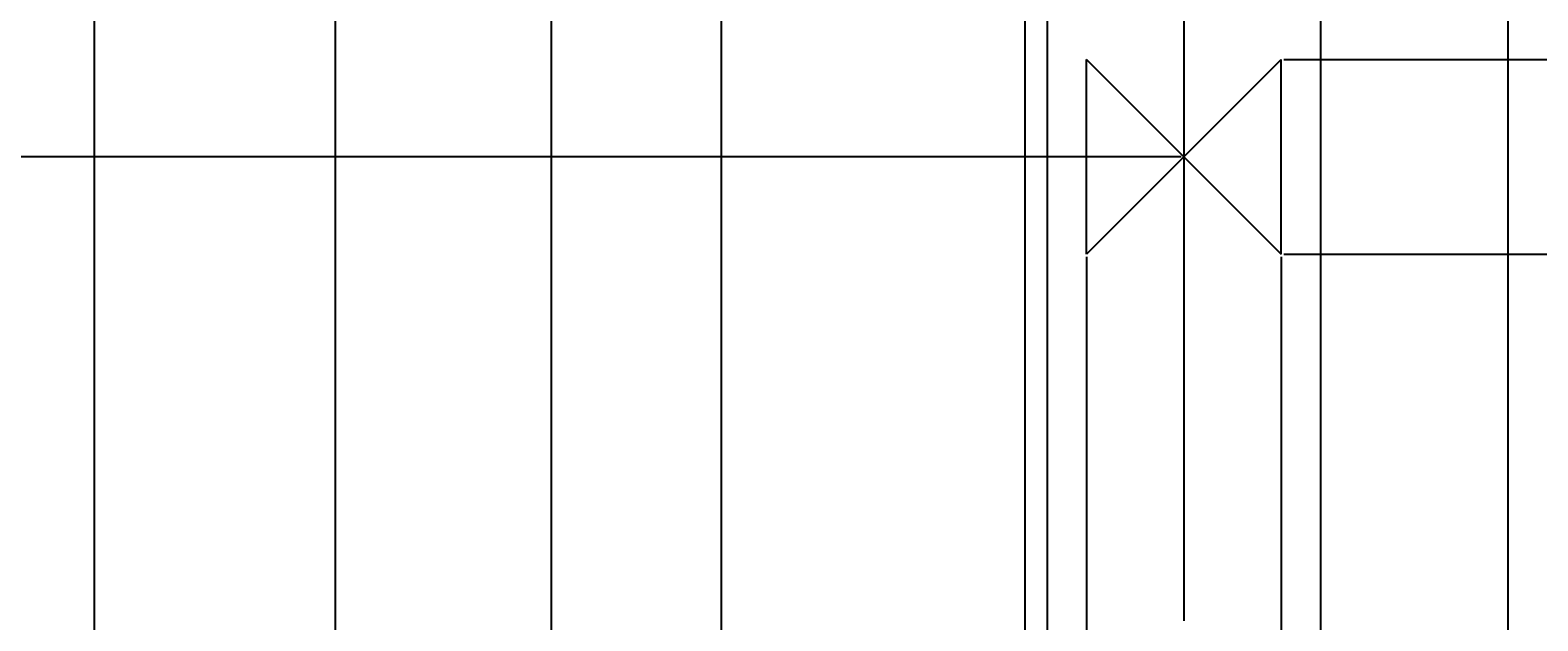
# Model space of a CAD drawing. Units: inches. Extents: x 412 to 584, y 208 to 437.
# Tile 18 of 28: x 471 to 508, y 338 to 352. Entities that reach past the tile are written whole.
import ezdxf

# ---------------------------------------------------------------- set-up
doc = ezdxf.new("R2010")
doc.units = ezdxf.units.IN
doc.header["$MEASUREMENT"] = 0
doc.layers.add('A-ANNO-DIMS', color=2, linetype='Continuous', lineweight=18)
doc.layers.add('E-POWR-EQPM', color=3, linetype='Continuous', lineweight=25)
doc.styles.get("Standard").update_dxf_attribs({"font": 'arial.ttf'})
doc.dimstyles.get("Standard").update_dxf_attribs({"dimtxt": 0.18, "dimasz": 0.18, "dimexe": 0.18, "dimexo": 0.0625, "dimgap": 0.09, "dimtad": 0, "dimtih": 1, "dimtoh": 1, "dimdec": 4, "dimzin": 0, "dimdsep": 46, "dimtxsty": 'Standard', "dimcen": 0.09, "dimadec": 0, "dimazin": 0, "dimtfac": 1, "dimtdec": 4, "dimtofl": 0, "dimtmove": 0, "dimatfit": 3, "dimfxl": 1, "dimtolj": 1, "dimtzin": 0, "dimarcsym": 0})

# ---------------------------------------------------------------- blocks, each defined once
blk = doc.blocks.new('*D17')
at = {"layer": 'A-ANNO-DIMS', "color": 0, "lineweight": -2, "transparency": 16777216}
for p, q in [((497.715, 426.185), (583.674, 426.185)), ((583.494, 426.005), (583.494, 323.031)), ((583.494, 219.693), (583.494, 322.667)), ((550.198, 219.513), (583.674, 219.513))]:
    blk.add_line(p, q, dxfattribs=at)
at = {"layer": 'A-ANNO-DIMS', "color": 0, "transparency": 16777216}
for points in [[(583.464, 426.005), (583.524, 426.005), (583.494, 426.185)], [(583.464, 219.693), (583.524, 219.693), (583.494, 219.513)]]:
    blk.add_solid(points, dxfattribs=at)
at = {"layer": 'Defpoints', "color": 0, "transparency": 16777216}
for p in [(497.652, 426.185), (550.135, 219.513), (583.494, 219.513)]:
    blk.add_point(p, dxfattribs=at)
at = {"layer": 'A-ANNO-DIMS', "color": 0, "transparency": 16777216, "insert": (583.494, 322.849), "char_height": 0.18, "attachment_point": 5}
blk.add_mtext('\\A1;206.67', dxfattribs=at)
blk = doc.blocks.new('*D23')
at = {"layer": 'A-ANNO-DIMS', "color": 0, "lineweight": -2, "transparency": 16777216}
for p, q in [((466.041, 360.196), (412.276, 360.196)), ((412.456, 360.016), (412.456, 354.967)), ((412.456, 349.553), (412.456, 354.603)), ((499.225, 349.373), (412.276, 349.373))]:
    blk.add_line(p, q, dxfattribs=at)
at = {"layer": 'A-ANNO-DIMS', "color": 0, "transparency": 16777216}
for points in [[(412.426, 360.016), (412.486, 360.016), (412.456, 360.196)], [(412.426, 349.553), (412.486, 349.553), (412.456, 349.373)]]:
    blk.add_solid(points, dxfattribs=at)
at = {"layer": 'Defpoints', "color": 0, "transparency": 16777216}
for p in [(466.104, 360.196), (412.456, 349.373), (499.288, 349.373)]:
    blk.add_point(p, dxfattribs=at)
at = {"layer": 'A-ANNO-DIMS', "color": 0, "transparency": 16777216, "insert": (412.456, 354.785), "char_height": 0.18, "attachment_point": 5}
blk.add_mtext('\\A1;10.823', dxfattribs=at)
blk = doc.blocks.new('*D24')
at = {"layer": 'A-ANNO-DIMS', "color": 0, "lineweight": -2, "transparency": 16777216}
for p, q in [((499.225, 349.373), (412.276, 349.373)), ((412.456, 349.193), (412.456, 340.743)), ((412.456, 331.93), (412.456, 340.38)), ((499.225, 331.75), (412.276, 331.75))]:
    blk.add_line(p, q, dxfattribs=at)
at = {"layer": 'A-ANNO-DIMS', "color": 0, "transparency": 16777216}
for points in [[(412.426, 349.193), (412.486, 349.193), (412.456, 349.373)], [(412.426, 331.93), (412.486, 331.93), (412.456, 331.75)]]:
    blk.add_solid(points, dxfattribs=at)
at = {"layer": 'Defpoints', "color": 0, "transparency": 16777216}
for p in [(499.288, 349.373), (412.456, 331.75), (499.288, 331.75)]:
    blk.add_point(p, dxfattribs=at)
at = {"layer": 'A-ANNO-DIMS', "color": 0, "transparency": 16777216, "insert": (412.456, 340.561), "char_height": 0.18, "attachment_point": 5}
blk.add_mtext('\\A1;17.624', dxfattribs=at)
blk = doc.blocks.new('*D28')
at = {"layer": 'A-ANNO-DIMS', "color": 0, "lineweight": -2, "transparency": 16777216}
for p, q in [((450.562, 256.635), (450.562, 437.465)), ((450.742, 437.285), (502.724, 437.285)), ((555.616, 437.285), (503.634, 437.285)), ((555.796, 256.635), (555.796, 437.465))]:
    blk.add_line(p, q, dxfattribs=at)
at = {"layer": 'A-ANNO-DIMS', "color": 0, "transparency": 16777216}
for points in [[(450.742, 437.315), (450.742, 437.255), (450.562, 437.285)], [(555.616, 437.315), (555.616, 437.255), (555.796, 437.285)]]:
    blk.add_solid(points, dxfattribs=at)
at = {"layer": 'Defpoints', "color": 0, "transparency": 16777216}
for p in [(555.796, 437.285), (450.562, 256.573), (555.796, 256.573)]:
    blk.add_point(p, dxfattribs=at)
at = {"layer": 'A-ANNO-DIMS', "color": 0, "transparency": 16777216, "insert": (503.179, 437.285), "char_height": 0.18, "attachment_point": 5}
blk.add_mtext('\\A1;105.23', dxfattribs=at)
blk = doc.blocks.new('*D29')
at = {"layer": 'A-ANNO-DIMS', "color": 0, "lineweight": -2, "transparency": 16777216}
for p, q in [((495.927, 378.924), (495.927, 208.233)), ((502.649, 378.924), (502.649, 208.233)), ((496.107, 208.413), (498.895, 208.413)), ((502.469, 208.413), (499.681, 208.413))]:
    blk.add_line(p, q, dxfattribs=at)
at = {"layer": 'A-ANNO-DIMS', "color": 0, "transparency": 16777216}
for points in [[(496.107, 208.443), (496.107, 208.383), (495.927, 208.413)], [(502.469, 208.443), (502.469, 208.383), (502.649, 208.413)]]:
    blk.add_solid(points, dxfattribs=at)
at = {"layer": 'Defpoints', "color": 0, "transparency": 16777216}
for p in [(495.927, 378.987), (502.649, 378.987), (502.649, 208.413)]:
    blk.add_point(p, dxfattribs=at)
at = {"layer": 'A-ANNO-DIMS', "color": 0, "transparency": 16777216, "insert": (499.288, 208.413), "char_height": 0.18, "attachment_point": 5}
blk.add_mtext('\\A1;6.722', dxfattribs=at)
blk = doc.blocks.new('*D31')
at = {"layer": 'A-ANNO-DIMS', "color": 0, "lineweight": -2, "transparency": 16777216}
for p, q in [((495.375, 405.385), (495.375, 208.233)), ((507.254, 405.385), (507.254, 208.233)), ((495.555, 208.413), (500.929, 208.413)), ((507.074, 208.413), (501.7, 208.413))]:
    blk.add_line(p, q, dxfattribs=at)
at = {"layer": 'A-ANNO-DIMS', "color": 0, "transparency": 16777216}
for points in [[(495.555, 208.443), (495.555, 208.383), (495.375, 208.413)], [(507.074, 208.443), (507.074, 208.383), (507.254, 208.413)]]:
    blk.add_solid(points, dxfattribs=at)
at = {"layer": 'Defpoints', "color": 0, "transparency": 16777216}
for p in [(495.375, 405.448), (507.254, 405.448), (507.254, 208.413)]:
    blk.add_point(p, dxfattribs=at)
at = {"layer": 'A-ANNO-DIMS', "color": 0, "transparency": 16777216, "insert": (501.314, 208.413), "char_height": 0.18, "attachment_point": 5}
blk.add_mtext('\\A1;11.88', dxfattribs=at)
blk = doc.blocks.new('*D33')
at = {"layer": 'A-ANNO-DIMS', "color": 0, "lineweight": -2, "transparency": 16777216}
for p, q in [((472.49, 363.226), (472.49, 208.233)), ((478.422, 363.226), (478.422, 208.233)), ((472.67, 208.413), (475.064, 208.413)), ((478.242, 208.413), (475.849, 208.413))]:
    blk.add_line(p, q, dxfattribs=at)
at = {"layer": 'A-ANNO-DIMS', "color": 0, "transparency": 16777216}
for points in [[(472.67, 208.443), (472.67, 208.383), (472.49, 208.413)], [(478.242, 208.443), (478.242, 208.383), (478.422, 208.413)]]:
    blk.add_solid(points, dxfattribs=at)
at = {"layer": 'Defpoints', "color": 0, "transparency": 16777216}
for p in [(472.49, 363.289), (478.422, 363.289), (478.422, 208.413)]:
    blk.add_point(p, dxfattribs=at)
at = {"layer": 'A-ANNO-DIMS', "color": 0, "transparency": 16777216, "insert": (475.456, 208.413), "char_height": 0.18, "attachment_point": 5}
blk.add_mtext('\\A1;5.932', dxfattribs=at)
blk = doc.blocks.new('*D39')
at = {"layer": 'A-ANNO-DIMS', "color": 0, "lineweight": -2, "transparency": 16777216}
for p, q in [((496.891, 346.914), (496.891, 208.233)), ((501.685, 346.914), (501.685, 208.233)), ((497.071, 208.413), (498.891, 208.413)), ((501.505, 208.413), (499.685, 208.413))]:
    blk.add_line(p, q, dxfattribs=at)
at = {"layer": 'A-ANNO-DIMS', "color": 0, "transparency": 16777216}
for points in [[(497.071, 208.443), (497.071, 208.383), (496.891, 208.413)], [(501.505, 208.443), (501.505, 208.383), (501.685, 208.413)]]:
    blk.add_solid(points, dxfattribs=at)
at = {"layer": 'Defpoints', "color": 0, "transparency": 16777216}
for p in [(496.891, 346.977), (501.685, 346.977), (501.685, 208.413)]:
    blk.add_point(p, dxfattribs=at)
at = {"layer": 'A-ANNO-DIMS', "color": 0, "transparency": 16777216, "insert": (499.288, 208.413), "char_height": 0.18, "attachment_point": 5}
blk.add_mtext('\\A1;4.794', dxfattribs=at)
blk = doc.blocks.new('*D40')
at = {"layer": 'A-ANNO-DIMS', "color": 0, "lineweight": -2, "transparency": 16777216}
for p, q in [((501.747, 351.77), (583.674, 351.77)), ((583.494, 351.59), (583.494, 349.555)), ((583.494, 347.157), (583.494, 349.191)), ((501.747, 346.977), (583.674, 346.977))]:
    blk.add_line(p, q, dxfattribs=at)
at = {"layer": 'A-ANNO-DIMS', "color": 0, "transparency": 16777216}
for points in [[(583.464, 351.59), (583.524, 351.59), (583.494, 351.77)], [(583.464, 347.157), (583.524, 347.157), (583.494, 346.977)]]:
    blk.add_solid(points, dxfattribs=at)
at = {"layer": 'Defpoints', "color": 0, "transparency": 16777216}
for p in [(501.685, 351.77), (501.685, 346.977), (583.494, 346.977)]:
    blk.add_point(p, dxfattribs=at)
at = {"layer": 'A-ANNO-DIMS', "color": 0, "transparency": 16777216, "insert": (583.494, 349.373), "char_height": 0.18, "attachment_point": 5}
blk.add_mtext('\\A1;4.794', dxfattribs=at)
blk = doc.blocks.new('*D41')
at = {"layer": 'A-ANNO-DIMS', "color": 0, "lineweight": -2, "transparency": 16777216}
for p, q in [((483.735, 316.045), (483.735, 437.465)), ((483.915, 437.285), (485.429, 437.285)), ((487.737, 437.285), (486.222, 437.285)), ((487.917, 316.045), (487.917, 437.465))]:
    blk.add_line(p, q, dxfattribs=at)
at = {"layer": 'A-ANNO-DIMS', "color": 0, "transparency": 16777216}
for points in [[(483.915, 437.315), (483.915, 437.255), (483.735, 437.285)], [(487.737, 437.315), (487.737, 437.255), (487.917, 437.285)]]:
    blk.add_solid(points, dxfattribs=at)
at = {"layer": 'Defpoints', "color": 0, "transparency": 16777216}
for p in [(487.917, 437.285), (483.735, 315.982), (487.917, 315.982)]:
    blk.add_point(p, dxfattribs=at)
at = {"layer": 'A-ANNO-DIMS', "color": 0, "transparency": 16777216, "insert": (485.826, 437.285), "char_height": 0.18, "attachment_point": 5}
blk.add_mtext('\\A1;4.182', dxfattribs=at)

msp = doc.modelspace()

# ---------------------------------------------------------------- linework, layer by layer
at = {"layer": 'E-POWR-EQPM'}
for p, q in [((499.2878, 358.9229), (499.2878, 349.3734)), ((499.2878, 349.3734), (496.891, 351.7702)), ((496.891, 346.9765), (496.891, 351.7702)), ((499.2878, 349.3734), (501.6846, 351.7702)), ((501.6846, 346.9765), (501.6846, 351.7702)), ((499.2878, 349.3734), (496.891, 346.9765)), ((499.2878, 349.3734), (501.6846, 346.9765)), ((499.2878, 349.3734), (499.2878, 337.9617))]:
    msp.add_line(p, q, dxfattribs=at)

# ---------------------------------------------------------------- dimensions: what is measured, and where the dimension line sits
at = {"layer": 'A-ANNO-DIMS'}
for base, p1, p2, override, picture, middle in [((555.7959, 437.2847), (450.562, 256.5729), (555.7959, 256.5729), {"dimdec": 2, "dimlfac": 1, "dimrnd": 0, "dimzin": 0, "dimdsep": 46, "dimlunit": 2}, '*D28', (503.1789, 437.2847)), ((487.9167, 437.2847), (483.7347, 315.9821), (487.9167, 315.9821), {"dimdec": 3, "dimlfac": 1, "dimrnd": 0, "dimzin": 0, "dimdsep": 46, "dimlunit": 2}, '*D41', (485.8257, 437.2847)), ((507.2538, 208.4133), (495.3746, 405.448), (507.2538, 405.448), {"dimdec": 2, "dimlfac": 1, "dimrnd": 0, "dimzin": 0, "dimdsep": 46, "dimlunit": 2}, '*D31', (501.3142, 208.4133)), ((502.6489, 208.4133), (495.9268, 378.9867), (502.6489, 378.9867), {"dimdec": 3, "dimlfac": 1, "dimrnd": 0, "dimzin": 0, "dimdsep": 46, "dimlunit": 2}, '*D29', (499.2878, 208.4133)), ((478.4225, 208.4133), (472.4903, 363.2888), (478.4225, 363.2888), {"dimdec": 3, "dimlfac": 1, "dimrnd": 0, "dimzin": 0, "dimdsep": 46, "dimlunit": 2}, '*D33', (475.4564, 208.4133)), ((501.6846, 208.4133), (496.891, 346.9765), (501.6846, 346.9765), {"dimdec": 3, "dimlfac": 1, "dimrnd": 0, "dimzin": 0, "dimdsep": 46, "dimlunit": 2}, '*D39', (499.2878, 208.4133))]:
    dim = msp.add_linear_dim(base=base, p1=p1, p2=p2, dimstyle='Standard', override=override, dxfattribs=at)
    dim.commit()
    dim.dimension.update_dxf_attribs({"geometry": picture, "text_midpoint": middle})
for base, p1, p2, override, picture, middle in [((583.4937, 219.5133), (497.6523, 426.1847), (550.1351, 219.5133), {"dimdec": 2, "dimlfac": 1, "dimrnd": 0, "dimzin": 0, "dimdsep": 46, "dimlunit": 2}, '*D17', (583.4937, 322.849)), ((412.4562, 349.3734), (466.1037, 360.1961), (499.2878, 349.3734), {"dimdec": 3, "dimlfac": 1, "dimrnd": 0, "dimzin": 0, "dimdsep": 46, "dimlunit": 2}, '*D23', (412.4562, 354.7847)), ((583.4937, 346.9765), (501.6846, 351.7702), (501.6846, 346.9765), {"dimdec": 3, "dimlfac": 1, "dimrnd": 0, "dimzin": 0, "dimdsep": 46, "dimlunit": 2}, '*D40', (583.4937, 349.3734)), ((412.4562, 331.7496), (499.2878, 349.3734), (499.2878, 331.7496), {"dimdec": 3, "dimlfac": 1, "dimrnd": 0, "dimzin": 0, "dimdsep": 46, "dimlunit": 2}, '*D24', (412.4562, 340.5615))]:
    dim = msp.add_linear_dim(base=base, p1=p1, p2=p2, angle=90, dimstyle='Standard', override=override, dxfattribs=at)
    dim.commit()
    dim.dimension.update_dxf_attribs({"geometry": picture, "text_midpoint": middle})

doc.saveas('drawing.dxf')
